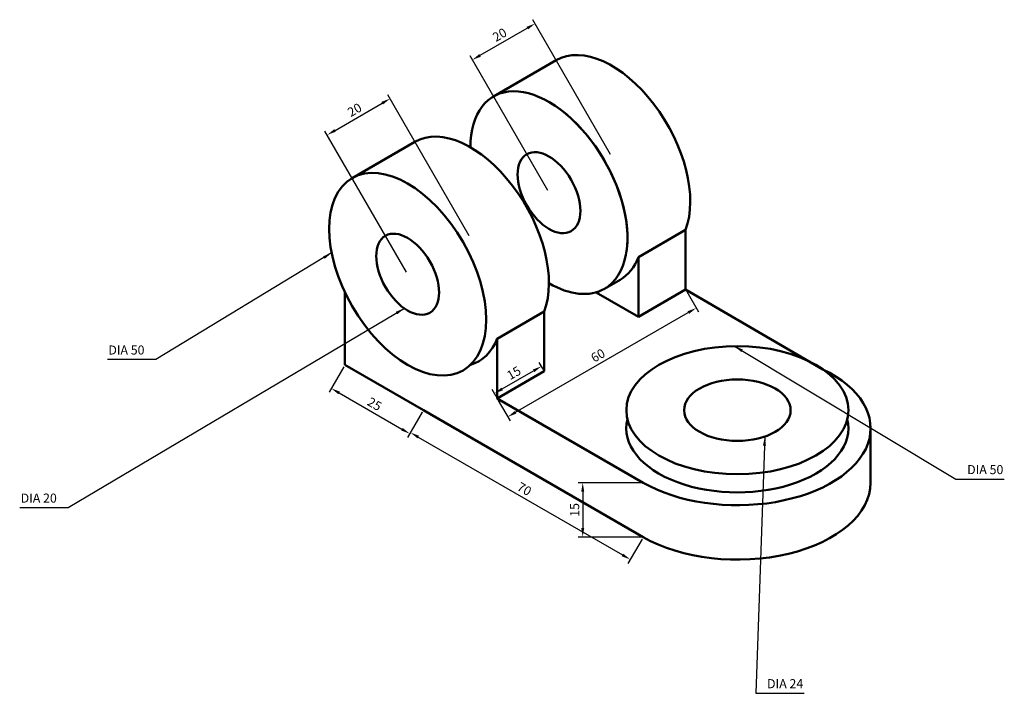
# Model space of a CAD drawing. Units: millimetres. Extents: x 2477 to 2749, y 1232 to 1417.
import ezdxf

# ---------------------------------------------------------------- set-up
doc = ezdxf.new("R2010")
doc.units = ezdxf.units.MM
for name, color, linetype, lineweight in [('M-DIMS', 2, 'Continuous', 25), ('M-OUTL', 7, 'Continuous', 50), ('M-TEXT', 3, 'Continuous', 25)]:
    doc.layers.add(name, color=color, linetype=linetype, lineweight=lineweight)
doc.styles.get("Standard").update_dxf_attribs({"font": 'arial.ttf'})
doc.dimstyles.new('ISO-25', dxfattribs={"dimtxt": 2.5, "dimasz": 2.5, "dimexe": 1.25, "dimexo": 0.625, "dimtad": 1, "dimtxsty": 'Standard', "dimcen": 2.5, "dimadec": 0, "dimazin": 0, "dimtfac": 1, "dimtmove": 0, "dimatfit": 3, "dimfxl": 1, "dimarcsym": 0})

# ---------------------------------------------------------------- blocks, each defined once
blk = doc.blocks.new('*D1')
at = {"layer": 'Defpoints', "color": 0, "transparency": 16777216}
for p in [(2660.78, 1342.86), (2663.71, 1337.79), (2608.82, 1312.86)]:
    blk.add_point(p, dxfattribs=at)
at = {"layer": 'M-DIMS', "color": 0, "lineweight": -2, "transparency": 16777216}
for p, q in [((2661.09, 1342.32), (2664.33, 1336.71)), ((2613.91, 1309.04), (2661.54, 1336.54)), ((2609.13, 1312.32), (2612.37, 1306.71))]:
    blk.add_line(p, q, dxfattribs=at)
at = {"layer": 'M-DIMS', "color": 0, "transparency": 16777216}
for points in [[(2661.33, 1336.9), (2661.75, 1336.18), (2663.71, 1337.79)], [(2613.7, 1309.4), (2614.12, 1308.68), (2611.75, 1307.79)]]:
    blk.add_solid(points, dxfattribs=at)
at = {"layer": 'M-DIMS', "color": 0, "transparency": 16777216, "insert": (2636.78, 1324.44), "char_height": 2.5, "attachment_point": 5, "rotation": 30}
blk.add_mtext('60', dxfattribs=at)
blk = doc.blocks.new('*D2')
at = {"layer": 'Defpoints', "color": 0, "transparency": 16777216}
for p in [(2566.81, 1322.12), (2588.46, 1309.62), (2584.72, 1303.13)]:
    blk.add_point(p, dxfattribs=at)
at = {"layer": 'M-DIMS', "color": 0, "lineweight": -2, "transparency": 16777216}
for p, q in [((2566.5, 1321.57), (2562.44, 1314.55)), ((2565.23, 1314.38), (2582.55, 1304.38)), ((2588.15, 1309.07), (2584.09, 1302.05))]:
    blk.add_line(p, q, dxfattribs=at)
at = {"layer": 'M-DIMS', "color": 0, "transparency": 16777216}
for points in [[(2565.44, 1314.74), (2565.02, 1314.02), (2563.07, 1315.63)], [(2582.76, 1304.74), (2582.34, 1304.02), (2584.72, 1303.13)]]:
    blk.add_solid(points, dxfattribs=at)
at = {"layer": 'M-DIMS', "color": 0, "transparency": 16777216, "insert": (2574.84, 1311.03), "char_height": 2.5, "attachment_point": 5, "rotation": 330}
blk.add_mtext('25', dxfattribs=at)
blk = doc.blocks.new('*D3')
at = {"layer": 'Defpoints', "color": 0, "transparency": 16777216}
for p in [(2588.46, 1309.62), (2649.08, 1274.62), (2645.52, 1268.45)]:
    blk.add_point(p, dxfattribs=at)
at = {"layer": 'M-DIMS', "color": 0, "lineweight": -2, "transparency": 16777216}
for p, q in [((2588.15, 1309.07), (2584.27, 1302.37)), ((2587.06, 1302.2), (2643.36, 1269.7)), ((2648.77, 1274.07), (2644.9, 1267.37))]:
    blk.add_line(p, q, dxfattribs=at)
at = {"layer": 'M-DIMS', "color": 0, "transparency": 16777216}
for points in [[(2587.27, 1302.56), (2586.86, 1301.84), (2584.9, 1303.45)], [(2643.56, 1270.06), (2643.15, 1269.34), (2645.52, 1268.45)]]:
    blk.add_solid(points, dxfattribs=at)
at = {"layer": 'M-DIMS', "color": 0, "transparency": 16777216, "insert": (2616.16, 1287.6), "char_height": 2.5, "attachment_point": 5, "rotation": 330}
blk.add_mtext('70', dxfattribs=at)
blk = doc.blocks.new('*D4')
at = {"layer": 'Defpoints', "color": 0, "transparency": 16777216}
for p in [(2579.27, 1395.53), (2601.45, 1357.12), (2584.13, 1347.12)]:
    blk.add_point(p, dxfattribs=at)
at = {"layer": 'M-DIMS', "color": 0, "lineweight": -2, "transparency": 16777216}
for p, q in [((2601.14, 1357.66), (2578.65, 1396.61)), ((2564.12, 1386.78), (2577.11, 1394.28)), ((2583.82, 1347.66), (2561.33, 1386.61))]:
    blk.add_line(p, q, dxfattribs=at)
at = {"layer": 'M-DIMS', "color": 0, "transparency": 16777216}
for points in [[(2576.9, 1394.64), (2577.32, 1393.92), (2579.27, 1395.53)], [(2563.91, 1387.14), (2564.32, 1386.42), (2561.95, 1385.53)]]:
    blk.add_solid(points, dxfattribs=at)
at = {"layer": 'M-DIMS', "color": 0, "transparency": 16777216, "insert": (2569.66, 1392.17), "char_height": 2.5, "attachment_point": 5, "rotation": 30}
blk.add_mtext('20', dxfattribs=at)
blk = doc.blocks.new('*D5')
at = {"layer": 'Defpoints', "color": 0, "transparency": 16777216}
for p in [(2619.28, 1416.23), (2640.42, 1379.62), (2623.1, 1369.62)]:
    blk.add_point(p, dxfattribs=at)
at = {"layer": 'M-DIMS', "color": 0, "lineweight": -2, "transparency": 16777216}
for p, q in [((2604.13, 1407.48), (2617.12, 1414.98)), ((2640.11, 1380.16), (2618.66, 1417.31)), ((2622.79, 1370.16), (2601.34, 1407.31))]:
    blk.add_line(p, q, dxfattribs=at)
at = {"layer": 'M-DIMS', "color": 0, "transparency": 16777216}
for points in [[(2616.91, 1415.34), (2617.33, 1414.61), (2619.28, 1416.23)], [(2603.92, 1407.84), (2604.34, 1407.11), (2601.96, 1406.23)]]:
    blk.add_solid(points, dxfattribs=at)
at = {"layer": 'M-DIMS', "color": 0, "transparency": 16777216, "insert": (2609.67, 1412.87), "char_height": 2.5, "attachment_point": 5, "rotation": 30}
blk.add_mtext('20', dxfattribs=at)
blk = doc.blocks.new('*D6')
at = {"layer": 'Defpoints', "color": 0, "transparency": 16777216}
for p in [(2621.02, 1321.72), (2621.81, 1320.36), (2608.82, 1312.86)]:
    blk.add_point(p, dxfattribs=at)
at = {"layer": 'M-DIMS', "color": 0, "lineweight": -2, "transparency": 16777216}
for p, q in [((2621.49, 1320.9), (2620.4, 1322.8)), ((2610.2, 1315.47), (2618.86, 1320.47)), ((2608.5, 1313.4), (2607.41, 1315.3))]:
    blk.add_line(p, q, dxfattribs=at)
at = {"layer": 'M-DIMS', "color": 0, "transparency": 16777216}
for points in [[(2618.65, 1320.83), (2619.07, 1320.11), (2621.02, 1321.72)], [(2609.99, 1315.83), (2610.41, 1315.11), (2608.03, 1314.22)]]:
    blk.add_solid(points, dxfattribs=at)
at = {"layer": 'M-DIMS', "color": 0, "transparency": 16777216, "insert": (2613.58, 1319.61), "char_height": 2.5, "attachment_point": 5, "rotation": 30}
blk.add_mtext('15', dxfattribs=at)
blk = doc.blocks.new('*D7')
at = {"layer": 'Defpoints', "color": 0, "transparency": 16777216}
for p in [(2649.08, 1289.62), (2632.41, 1274.62), (2649.08, 1274.62)]:
    blk.add_point(p, dxfattribs=at)
at = {"layer": 'M-DIMS', "color": 0, "lineweight": -2, "transparency": 16777216}
for p, q in [((2648.45, 1289.62), (2631.16, 1289.62)), ((2632.41, 1287.12), (2632.41, 1277.12)), ((2648.45, 1274.62), (2631.16, 1274.62))]:
    blk.add_line(p, q, dxfattribs=at)
at = {"layer": 'M-DIMS', "color": 0, "transparency": 16777216}
for points in [[(2632, 1287.12), (2632.83, 1287.12), (2632.41, 1289.62)], [(2632, 1277.12), (2632.83, 1277.12), (2632.41, 1274.62)]]:
    blk.add_solid(points, dxfattribs=at)
at = {"layer": 'M-DIMS', "color": 0, "transparency": 16777216, "insert": (2630.51, 1282.12), "char_height": 2.5, "attachment_point": 5, "rotation": 90}
blk.add_mtext('15', dxfattribs=at)

msp = doc.modelspace()

# ---------------------------------------------------------------- linework, layer by layer
at = {"layer": 'M-OUTL'}
for p, q in [((2607.79, 1396.132), (2625.11, 1406.132)), ((2568.819, 1373.632), (2586.139, 1383.632)), ((2647.781, 1351.836), (2660.771, 1359.336)), ((2660.771, 1342.866), (2660.771, 1359.336)), ((2647.781, 1335.366), (2647.781, 1351.836)), ((2638.408, 1343.099), (2642.739, 1345.599)), ((2566.808, 1322.116), (2566.808, 1342.116)), ((2647.781, 1335.366), (2636.09, 1342.116)), ((2647.781, 1335.366), (2660.771, 1342.866)), ((2698.679, 1320.866), (2660.778, 1342.862)), ((2608.81, 1329.336), (2621.8, 1336.836)), ((2621.807, 1320.362), (2621.807, 1336.854)), ((2608.817, 1312.862), (2608.817, 1329.354)), ((2588.458, 1309.616), (2566.808, 1322.116)), ((2608.817, 1312.862), (2621.807, 1320.362)), ((2649.08, 1289.616), (2608.817, 1312.862)), ((2588.458, 1309.616), (2649.08, 1274.616)), ((2711.803, 1304.616), (2711.803, 1289.616))]:
    msp.add_line(p, q, dxfattribs=at)
for centre, major_axis, start_param, end_param in [((2640.42, 1379.616), (15.309, -26.517), 6.7213343, 9.424778), ((2623.099, 1369.616), (15.309, -26.517), 6.9103422, 10.2101761), ((2623.099, 1369.616), (15.309, -26.517), 0, 2.3561945), ((2601.449, 1357.116), (15.309, -26.517), 6.7213343, 9.424778), ((2627.429, 1372.116), (15.309, -26.517), 0, 0.4372321), ((2623.099, 1369.616), (15.309, -26.517), 5.4977871, 6.2831853), ((2588.458, 1349.616), (15.309, -26.517), 6.1412883, 6.7213343), ((2675.061, 1304.616), (-36.742, 0), 7.0685835, 10.2974238), ((2675.061, 1304.616), (-30.619, 0), 6.1412883, 9.566675), ((2675.061, 1289.616), (-36.742, 0), 7.0685835, 9.424778)]:
    msp.add_ellipse(centre, major_axis=major_axis, ratio=0.5773503, start_param=start_param, end_param=end_param, dxfattribs=at)
for centre, major_axis in [((2623.099, 1369.616), (6.124, -10.607)), ((2584.128, 1347.116), (15.309, -26.517)), ((2584.128, 1347.116), (6.124, -10.607)), ((2675.061, 1309.616), (-30.619, 0)), ((2675.061, 1309.616), (-14.697, 0))]:
    msp.add_ellipse(centre, major_axis=major_axis, ratio=0.5773503, dxfattribs=at)

# ---------------------------------------------------------------- texts
at = {"layer": 'M-TEXT', "char_height": 2.5}
for s, insert, attachment_point in [('DIA 50', (2511.55, 1324.186), 9), ('DIA 50', (2738.446, 1291.2), 7), ('DIA 20', (2487.371, 1283.34), 9), ('DIA 24', (2683.257, 1232.162), 7)]:
    msp.add_mtext(s, dxfattribs=dict(at, insert=insert, attachment_point=attachment_point))

# ---------------------------------------------------------------- dimensions: what is measured, and where the dimension line sits
at = {"layer": 'M-DIMS'}
for p1, p2, distance, picture, middle in [((2623.099, 1369.616), (2640.42, 1379.616), 42.273, '*D5', (2609.672, 1412.872)), ((2584.128, 1347.116), (2601.449, 1357.116), 44.354, '*D4', (2569.661, 1392.174)), ((2608.817, 1312.862), (2660.778, 1342.862), -5.858, '*D1', (2636.775, 1324.436)), ((2608.817, 1312.862), (2621.807, 1320.362), 1.566, '*D6', (2613.578, 1319.614)), ((2566.808, 1322.116), (2588.458, 1309.616), -7.485, '*D2', (2574.841, 1311.031)), ((2588.458, 1309.616), (2649.08, 1274.616), -7.117, '*D3', (2616.161, 1287.599)), ((2649.08, 1289.616), (2649.08, 1274.616), -16.667, '*D7', (2630.512, 1282.116))]:
    dim = msp.add_aligned_dim(p1=p1, p2=p2, distance=distance, dimstyle='ISO-25', override={"dimclrd": 0, "dimclre": 0, "dimclrt": 0}, dxfattribs=at)
    dim.commit()
    dim.dimension.update_dxf_attribs({"geometry": picture, "text_midpoint": middle})

# ---------------------------------------------------------------- leaders
at = {"layer": 'M-TEXT', "annotation_type": 0, "has_hookline": 1}
for points, hookline_direction, text_width in [([(2563.159, 1352.997), (2514.675, 1323.561), (2512.175, 1323.561)], 1, 10.24), ([(2583.222, 1337.694), (2490.496, 1282.715), (2487.996, 1282.715)], 1, 10.24), ([(2674.234, 1327.287), (2735.321, 1290.575), (2737.821, 1290.575)], 0, 10.24), ([(2682.632, 1302.343), (2680.132, 1231.537), (2682.632, 1231.537)], 0, 10.239)]:
    msp.add_leader(points, dimstyle='ISO-25', dxfattribs=dict(at, hookline_direction=hookline_direction, text_width=text_width))

doc.saveas('drawing.dxf')
